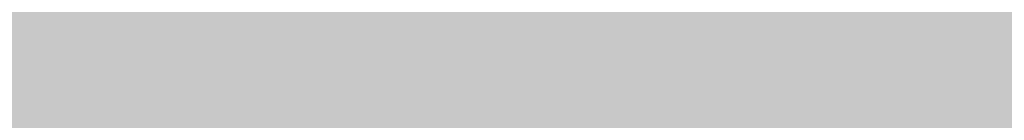
# Model space of a CAD drawing. Units: feet. Extents: x 3168 to 4724, y 827 to 1477.
# Tile 205 of 256: x 3333 to 3364, y 1094 to 1097. Entities that reach past the tile are written whole.
import ezdxf

# ---------------------------------------------------------------- set-up
doc = ezdxf.new("R2010")
doc.units = ezdxf.units.FT
doc.layers.add('A-ELEV-PATT', color=8, linetype='Continuous', lineweight=13)

msp = doc.modelspace()

# ---------------------------------------------------------------- hatches: boundary and pattern name
at = {"layer": 'A-ELEV-PATT'}
h = msp.add_hatch(color=256, dxfattribs=at)
h.dxf.hatch_style = 1
edge = h.paths.add_edge_path()
edge.add_ellipse((3552.906, 979.22), major_axis=(36.745, 0), ratio=0.484848, start_angle=0, end_angle=360)
edge = h.paths.add_edge_path()
edge.add_ellipse((3559.892, 929.252), major_axis=(36.745, 0), ratio=0.484848, start_angle=0, end_angle=360)
edge = h.paths.add_edge_path()
edge.add_line((3299.317, 1198.606), (3479.917, 1198.606))
edge.add_line((3479.917, 1198.606), (3479.917, 1209.869))
edge.add_spline(control_points=[(3479.917, 1209.869), (3464.301, 1209.869), (3448.686, 1209.869), (3410.949, 1209.869), (3388.828, 1209.869), (3355.647, 1209.869), (3344.586, 1209.869), (3327.996, 1209.869), (3322.466, 1209.869), (3314.17, 1209.869), (3311.405, 1209.869), (3307.257, 1209.869), (3305.875, 1209.869), (3303.801, 1209.869), (3303.11, 1209.869), (3302.073, 1209.869), (3301.727, 1209.869), (3301.209, 1209.869), (3301.036, 1209.869), (3300.777, 1209.869), (3300.69, 1209.869), (3300.561, 1209.869), (3300.517, 1209.869), (3300.453, 1209.869), (3300.431, 1209.869), (3300.399, 1209.869), (3300.388, 1209.869), (3300.366, 1209.869), (3300.346, 1209.869), (3300.346, 1209.869), (3300.346, 1209.869), (3300.343, 1209.869), (3300.341, 1209.869), (3300.338, 1209.869), (3300.337, 1209.869), (3300.334, 1209.869), (3300.332, 1209.869), (3300.326, 1209.869), (3300.321, 1209.869), (3300.311, 1209.869), (3300.306, 1209.869), (3300.291, 1209.869), (3300.28, 1209.869), (3300.232, 1209.869), (3300.195, 1209.869), (3299.951, 1209.871), (3299.745, 1209.874), (3299.437, 1209.883), (3299.334, 1209.887), (3299.181, 1209.893), (3299.13, 1209.895), (3298.652, 1209.917), (3298.229, 1209.946), (3297.602, 1210.002), (3297.393, 1210.023), (3297.083, 1210.058), (3296.979, 1210.07), (3296.293, 1210.155), (3295.718, 1210.243), (3294.869, 1210.399), (3294.588, 1210.454), (3294.169, 1210.543), (3294.03, 1210.574), (3291.707, 1211.101), (3289.654, 1211.813), (3285.776, 1213.564), (3283.951, 1214.603), (3280.512, 1216.98), (3278.897, 1218.318), (3276.38, 1220.829), (3275.416, 1221.918), (3274.039, 1223.708), (3273.581, 1224.35), (3273.143, 1225.016)], knot_values=[39.119033, 39.119033, 39.119033, 39.119033, 39.286353, 39.286353, 39.523379, 39.523379, 39.641892, 39.641892, 39.701148, 39.701148, 39.730777, 39.730777, 39.745591, 39.745591, 39.752998, 39.752998, 39.756701, 39.756701, 39.758553, 39.758553, 39.759479, 39.759479, 39.759942, 39.759942, 39.760173, 39.760173, 39.760289, 39.760289, 39.760405, 39.760405, 39.760463, 39.760463, 39.763389, 39.763389, 39.764851, 39.764851, 39.767304, 39.767304, 39.773825, 39.773825, 39.78057, 39.78057, 39.79477, 39.79477, 39.845194, 39.845194, 40.126715, 40.126715, 40.267476, 40.267476, 40.337856, 40.337856, 40.927023, 40.927023, 41.221606, 41.221606, 41.368898, 41.368898, 42.202622, 42.202622, 42.619485, 42.619485, 42.827916, 42.827916, 46.118323, 46.118323, 49.408731, 49.408731, 52.699139, 52.699139, 54.927489, 54.927489, 56.104228, 56.104228, 56.104228, 56.104228], weights=[1, 1, 1, 1, 1, 1, 1, 1, 1, 1, 1, 1, 1, 1, 1, 1, 1, 1, 1, 1, 1, 1, 1, 1, 1, 1, 1, 1, 1, 1, 1, 1, 1, 1, 1, 1, 1, 1, 1, 1, 1, 1, 1, 1, 1, 1, 1, 1, 1, 1, 1, 1, 1, 1, 1, 1, 1, 1, 1, 1, 1, 1, 1, 1, 1, 1, 1, 1, 1, 1, 1, 1, 1, 1], degree=3, periodic=0)
edge.add_line((3273.143, 1225.016), (3273.143, 1099.016))
edge.add_line((3273.143, 1099.016), (3299.317, 1099.016))
edge.add_line((3299.317, 1099.016), (3299.317, 1198.606))
edge = h.paths.add_edge_path()
edge.add_line((3304.758, 1324.158), (3479.917, 1324.158))
edge.add_line((3479.917, 1324.158), (3479.917, 1335.715))
edge.add_line((3479.917, 1335.715), (3269.162, 1335.715))
edge.add_spline(control_points=[(3269.162, 1335.715), (3264.024, 1335.715), (3258.364, 1328.958), (3259.264, 1323.9)], knot_values=[0, 0, 0, 0, 15.412191, 15.412191, 15.412191, 15.412191], degree=3, periodic=0)
edge.add_line((3259.264, 1323.9), (3265.517, 1288.769))
edge.add_line((3265.517, 1288.769), (3275.265, 1261.546))
edge.add_line((3275.265, 1261.546), (3304.758, 1261.546))
edge.add_line((3304.758, 1261.546), (3304.758, 1324.158))
h = msp.add_hatch(color=256, dxfattribs=at)
h.dxf.hatch_style = 1
h.paths.add_polyline_path([(3384.525, 1099.016), (3335.029, 1099.016), (3299.317, 1099.016), (3273.143, 1099.016), (3217.565, 1099.016), (3168.069, 827.116), (3335.029, 827.116)])

doc.saveas('drawing.dxf')
